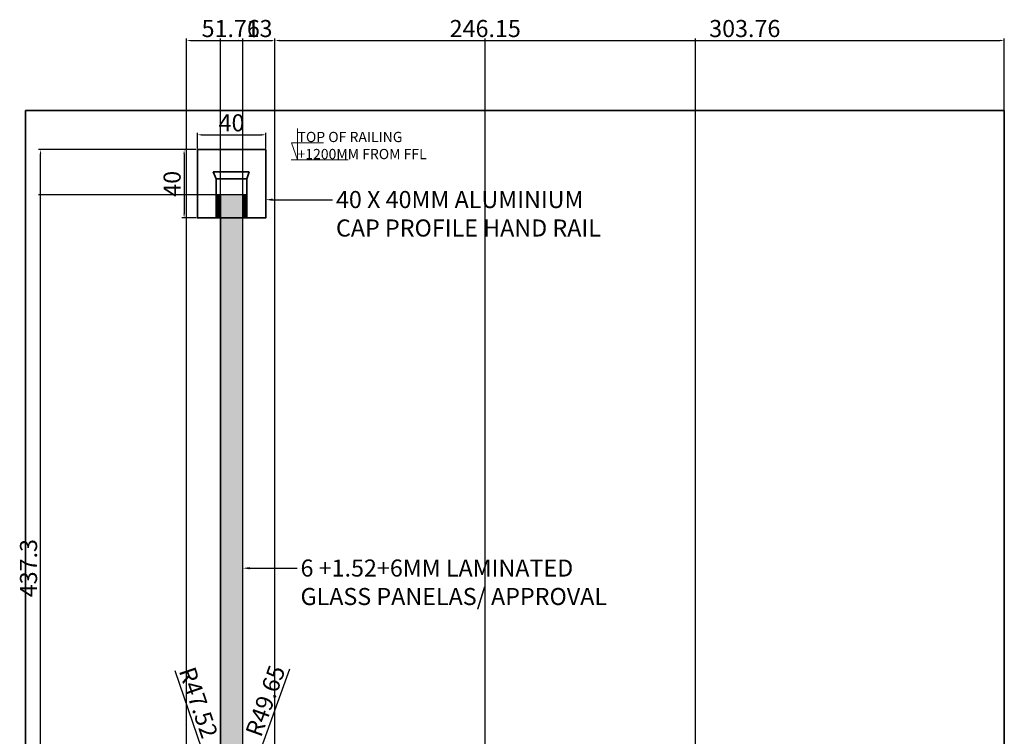
# Model space of a CAD drawing. Units: millimetres. Extents: x 1791 to 2420, y 1225 to 2361.
# Tile 4 of 4: x 1791 to 2367, y 1941 to 2361. Entities that reach past the tile are written whole.
import ezdxf
from ezdxf import colors
from ezdxf.entities.mleader import LeaderData, LeaderLine
from ezdxf.math import Vec2, Vec3

# ---------------------------------------------------------------- set-up
doc = ezdxf.new("R2010")
doc.units = ezdxf.units.MM
for name, color, linetype, lineweight in [('A-ANNO-DIMS', 2, 'Continuous', 18), ('A-ANNO-SYMB', 7, 'Continuous', 18), ('A-ANNO-TEXT', 7, 'Continuous', 18), ('A-ANNO-TTLB', 7, 'Continuous', 35), ('A-DETL-PATT', 8, 'Continuous', 13), ('A-GLAZ', 5, 'Continuous', 25), ('A-RAIL', 4, 'Continuous', 35)]:
    doc.layers.add(name, color=color, linetype=linetype, lineweight=lineweight)
doc.styles.get("Standard").update_dxf_attribs({"font": 'arial.ttf'})
doc.dimstyles.new('ISO-25', dxfattribs={"dimtxt": 10, "dimasz": 2.5, "dimexe": 1.25, "dimexo": 0.625, "dimtad": 1, "dimdec": 1, "dimtxsty": 'Standard', "dimcen": 2.5, "dimadec": 0, "dimazin": 0, "dimtfac": 1, "dimtdec": 1, "dimtmove": 0, "dimatfit": 3, "dimfxl": 1, "dimarcsym": 0})

# ---------------------------------------------------------------- blocks, each defined once
blk = doc.blocks.new('*D1')
at = {"layer": 'A-ANNO-DIMS', "color": 0, "lineweight": -2, "transparency": 16777216}
for p, q in [((1895, 2285.61), (1895, 2294.91)), ((1897.5, 2293.66), (1932.5, 2293.66)), ((1935, 2285.61), (1935, 2294.91))]:
    blk.add_line(p, q, dxfattribs=at)
at = {"layer": 'A-ANNO-DIMS', "color": 0, "transparency": 16777216}
for points in [[(1897.5, 2294.08), (1897.5, 2293.25), (1895, 2293.66)], [(1932.5, 2294.08), (1932.5, 2293.25), (1935, 2293.66)]]:
    blk.add_solid(points, dxfattribs=at)
at = {"layer": 'Defpoints', "color": 0, "transparency": 16777216}
for p in [(1935, 2293.66), (1895, 2284.98), (1935, 2284.98)]:
    blk.add_point(p, dxfattribs=at)
at = {"layer": 'A-ANNO-DIMS', "color": 0, "transparency": 16777216, "insert": (1915, 2299.39), "char_height": 10, "attachment_point": 5}
blk.add_mtext('40', dxfattribs=at)
blk = doc.blocks.new('*D2')
at = {"layer": 'A-ANNO-DIMS', "color": 0, "lineweight": -2, "transparency": 16777216}
for p, q in [((1894.37, 2284.98), (1885.99, 2284.98)), ((1887.24, 2282.48), (1887.24, 2247.48)), ((1894.37, 2244.98), (1885.99, 2244.98))]:
    blk.add_line(p, q, dxfattribs=at)
at = {"layer": 'A-ANNO-DIMS', "color": 0, "transparency": 16777216}
for points in [[(1886.82, 2282.48), (1887.66, 2282.48), (1887.24, 2284.98)], [(1886.82, 2247.48), (1887.66, 2247.48), (1887.24, 2244.98)]]:
    blk.add_solid(points, dxfattribs=at)
at = {"layer": 'Defpoints', "color": 0, "transparency": 16777216}
for p in [(1895, 2284.98), (1887.24, 2244.98), (1895, 2244.98)]:
    blk.add_point(p, dxfattribs=at)
at = {"layer": 'A-ANNO-DIMS', "color": 0, "transparency": 16777216, "insert": (1881.51, 2264.98), "char_height": 10, "attachment_point": 5, "rotation": 90}
blk.add_mtext('40', dxfattribs=at)
blk = doc.blocks.new('*D11')
at = {"layer": 'A-ANNO-DIMS', "color": 0, "lineweight": -2, "transparency": 16777216}
for p, q in [((1894.37, 2284.98), (1801.98, 2284.98)), ((1803.23, 1317.92), (1803.23, 2282.48)), ((1854.1, 1315.42), (1801.98, 1315.42))]:
    blk.add_line(p, q, dxfattribs=at)
at = {"layer": 'A-ANNO-DIMS', "color": 0, "transparency": 16777216}
for points in [[(1802.81, 2282.48), (1803.64, 2282.48), (1803.23, 2284.98)], [(1802.81, 1317.92), (1803.64, 1317.92), (1803.23, 1315.42)]]:
    blk.add_solid(points, dxfattribs=at)
at = {"layer": 'Defpoints', "color": 0, "transparency": 16777216}
for p in [(1803.23, 2284.98), (1895, 2284.98), (1854.73, 1315.42)]:
    blk.add_point(p, dxfattribs=at)
at = {"layer": 'A-ANNO-DIMS', "color": 0, "transparency": 16777216, "insert": (1797.5, 1800.2), "char_height": 10, "attachment_point": 5, "rotation": 90}
blk.add_mtext('969.6', dxfattribs=at)
blk = doc.blocks.new('*D12')
at = {"layer": 'A-ANNO-DIMS', "color": 0, "lineweight": -2, "transparency": 16777216}
for p, q in [((1908.56, 1821.87), (1908.56, 2350.12)), ((1911.06, 2348.87), (1919.06, 2348.87)), ((1921.56, 1821.87), (1921.56, 2350.12)), ((1921.56, 2348.87), (1938.7, 2348.87))]:
    blk.add_line(p, q, dxfattribs=at)
at = {"layer": 'A-ANNO-DIMS', "color": 0, "transparency": 16777216}
for points in [[(1911.06, 2349.29), (1911.06, 2348.45), (1908.56, 2348.87)], [(1919.06, 2349.29), (1919.06, 2348.45), (1921.56, 2348.87)]]:
    blk.add_solid(points, dxfattribs=at)
at = {"layer": 'Defpoints', "color": 0, "transparency": 16777216}
for p in [(1921.56, 2348.87), (1908.56, 1821.24), (1921.56, 1821.24)]:
    blk.add_point(p, dxfattribs=at)
at = {"layer": 'A-ANNO-DIMS', "color": 0, "transparency": 16777216, "insert": (1931.38, 2354.6), "char_height": 10, "attachment_point": 5}
blk.add_mtext('13', dxfattribs=at)
blk = doc.blocks.new('*D13')
at = {"layer": 'A-ANNO-DIMS', "color": 0, "lineweight": -2, "transparency": 16777216}
for p, q in [((1907.94, 2258.52), (1801.98, 2258.52)), ((1803.23, 1823.74), (1803.23, 2256.02)), ((1907.94, 1821.24), (1801.98, 1821.24))]:
    blk.add_line(p, q, dxfattribs=at)
at = {"layer": 'A-ANNO-DIMS', "color": 0, "transparency": 16777216}
for points in [[(1802.81, 2256.02), (1803.64, 2256.02), (1803.23, 2258.52)], [(1802.81, 1823.74), (1803.64, 1823.74), (1803.23, 1821.24)]]:
    blk.add_solid(points, dxfattribs=at)
at = {"layer": 'Defpoints', "color": 0, "transparency": 16777216}
for p in [(1803.23, 2258.52), (1908.56, 2258.52), (1908.56, 1821.24)]:
    blk.add_point(p, dxfattribs=at)
at = {"layer": 'A-ANNO-DIMS', "color": 0, "transparency": 16777216, "insert": (1797.49, 2039.88), "char_height": 10, "attachment_point": 5, "rotation": 90}
blk.add_mtext('437.3', dxfattribs=at)
blk = doc.blocks.new('*D15')
at = {"layer": 'A-ANNO-DIMS', "color": 0, "lineweight": -2, "transparency": 16777216}
for p, q in [((1888.61, 1928.05), (1888.61, 2350.12)), ((1891.11, 2348.87), (1937.88, 2348.87)), ((1940.38, 1928.05), (1940.38, 2350.12))]:
    blk.add_line(p, q, dxfattribs=at)
at = {"layer": 'A-ANNO-DIMS', "color": 0, "transparency": 16777216}
for points in [[(1891.11, 2349.29), (1891.11, 2348.45), (1888.61, 2348.87)], [(1937.88, 2349.29), (1937.88, 2348.45), (1940.38, 2348.87)]]:
    blk.add_solid(points, dxfattribs=at)
at = {"layer": 'Defpoints', "color": 0, "transparency": 16777216}
for p in [(1940.38, 2348.87), (1888.61, 1927.42), (1940.38, 1927.42)]:
    blk.add_point(p, dxfattribs=at)
at = {"layer": 'A-ANNO-DIMS', "color": 0, "transparency": 16777216, "insert": (1914.5, 2354.6), "char_height": 10, "attachment_point": 5}
blk.add_mtext('51.76', dxfattribs=at)
blk = doc.blocks.new('*D27')
at = {"layer": 'A-ANNO-DIMS', "color": 0, "lineweight": -2, "transparency": 16777216}
for p, q in [((1940.38, 1808.78), (1940.38, 2350.12)), ((1942.88, 2348.87), (2184.03, 2348.87)), ((2186.53, 1808.78), (2186.53, 2350.12))]:
    blk.add_line(p, q, dxfattribs=at)
at = {"layer": 'A-ANNO-DIMS', "color": 0, "transparency": 16777216}
for points in [[(1942.88, 2349.29), (1942.88, 2348.45), (1940.38, 2348.87)], [(2184.03, 2349.29), (2184.03, 2348.45), (2186.53, 2348.87)]]:
    blk.add_solid(points, dxfattribs=at)
at = {"layer": 'Defpoints', "color": 0, "transparency": 16777216}
for p in [(2186.53, 2348.87), (1940.38, 1808.15), (2186.53, 1808.15)]:
    blk.add_point(p, dxfattribs=at)
at = {"layer": 'A-ANNO-DIMS', "color": 0, "transparency": 16777216, "insert": (2063.45, 2354.6), "char_height": 10, "attachment_point": 5}
blk.add_mtext('246.15', dxfattribs=at)
blk = doc.blocks.new('*D28')
at = {"layer": 'A-ANNO-DIMS', "color": 0, "lineweight": -2, "transparency": 16777216}
for p, q in [((2063.45, 1837.62), (2063.45, 2350.12)), ((2065.95, 2348.87), (2364.72, 2348.87)), ((2367.22, 1837.62), (2367.22, 2350.12))]:
    blk.add_line(p, q, dxfattribs=at)
at = {"layer": 'A-ANNO-DIMS', "color": 0, "transparency": 16777216}
for points in [[(2065.95, 2349.29), (2065.95, 2348.45), (2063.45, 2348.87)], [(2364.72, 2349.29), (2364.72, 2348.45), (2367.22, 2348.87)]]:
    blk.add_solid(points, dxfattribs=at)
at = {"layer": 'Defpoints', "color": 0, "transparency": 16777216}
for p in [(2367.22, 2348.87), (2063.45, 1837), (2367.22, 1837)]:
    blk.add_point(p, dxfattribs=at)
at = {"layer": 'A-ANNO-DIMS', "color": 0, "transparency": 16777216, "insert": (2215.34, 2354.6), "char_height": 10, "attachment_point": 5}
blk.add_mtext('303.76', dxfattribs=at)
blk = doc.blocks.new('*D40')
at = {"layer": 'A-ANNO-DIMS', "color": 0, "lineweight": -2, "transparency": 16777216}
for p, q in [((1948.97, 1980.8), (1932.16, 1934.12)), ((1914.5, 1885.05), (1931.31, 1931.76))]:
    blk.add_line(p, q, dxfattribs=at)
at = {"layer": 'A-ANNO-DIMS', "color": 0, "transparency": 16777216}
blk.add_solid([(1931.77, 1934.26), (1932.55, 1933.98), (1931.31, 1931.76)], dxfattribs=at)
at = {"layer": 'Defpoints', "color": 0, "transparency": 16777216}
for p in [(1931.31, 1931.76), (1914.5, 1885.05)]:
    blk.add_point(p, dxfattribs=at)
at = {"layer": 'A-ANNO-DIMS', "color": 0, "transparency": 16777216, "insert": (1936.01, 1961.74), "char_height": 10, "attachment_point": 5, "rotation": 70.20087}
blk.add_mtext('R49.65', dxfattribs=at)
blk = doc.blocks.new('*D41')
at = {"layer": 'A-ANNO-DIMS', "color": 0, "lineweight": -2, "transparency": 16777216}
for p, q in [((1881.8, 1979.97), (1897.4, 1934.31)), ((1913.57, 1886.98), (1898.2, 1931.95))]:
    blk.add_line(p, q, dxfattribs=at)
at = {"layer": 'A-ANNO-DIMS', "color": 0, "transparency": 16777216}
blk.add_solid([(1897.79, 1934.45), (1897, 1934.18), (1898.2, 1931.95)], dxfattribs=at)
at = {"layer": 'Defpoints', "color": 0, "transparency": 16777216}
for p in [(1898.2, 1931.95), (1913.57, 1886.98)]:
    blk.add_point(p, dxfattribs=at)
at = {"layer": 'A-ANNO-DIMS', "color": 0, "transparency": 16777216, "insert": (1894.41, 1960.78), "char_height": 10, "attachment_point": 5, "rotation": 288.8663}
blk.add_mtext('R47.52', dxfattribs=at)

msp = doc.modelspace()

# ---------------------------------------------------------------- hatches: boundary and pattern name
at = {"layer": 'A-DETL-PATT'}
h = msp.add_hatch(dxfattribs=at)
h.set_pattern_fill('ANSI31', color=256, scale=0.2)
h.paths.add_polyline_path([(1924.019, 2258.5157), (1921.5621, 2258.5157), (1921.5621, 2244.9823), (1924.019, 2244.9823)])
h.paths.add_polyline_path([(1908.5621, 2258.5157), (1906.091, 2258.5157), (1906.091, 2244.9823), (1908.5621, 2244.9823)])
h = msp.add_hatch(color=256, dxfattribs=at)
h.dxf.hatch_style = 1
h.paths.add_polyline_path([(1921.5621, 2258.5157), (1908.5621, 2258.5157), (1908.5621, 1821.2446), (1921.5621, 1821.2446)])

# ---------------------------------------------------------------- linework, layer by layer
at = {"layer": 'A-ANNO-SYMB'}
for p, q in [((1953.6131, 2297.3684), (1953.6131, 2279.0845)), ((1950.0667, 2289.0383), (1968.711, 2289.0383)), ((1953.6131, 2279.0791), (1950.0667, 2289.0383)), ((1949.9706, 2279.0845), (1983.1824, 2279.0845))]:
    msp.add_line(p, q, dxfattribs=at)
at = {"layer": 'A-ANNO-TTLB'}
for p, q in [((1794.3467, 1287.0028), (1794.3467, 2307.8191)), ((1794.3467, 2307.8191), (2367.2176, 2307.8191)), ((2367.2176, 2307.8191), (2367.2176, 1287.0028))]:
    msp.add_line(p, q, dxfattribs=at)
at = {"layer": 'A-GLAZ'}
msp.add_lwpolyline([(1908.5621, 1821.2446), (1921.5621, 1821.2446), (1921.5621, 2258.5157), (1908.5621, 2258.5157)], close=True, dxfattribs=at)
at = {"layer": 'A-RAIL'}
for p, q in [((1904.2456, 2272.0222), (1925.3645, 2272.0222)), ((1906.091, 2267.8964), (1904.2456, 2272.0222)), ((1924.019, 2267.8964), (1925.3645, 2272.0222)), ((1908.5621, 2258.5157), (1906.091, 2258.5157)), ((1921.5621, 2258.5157), (1924.019, 2258.5157))]:
    msp.add_line(p, q, dxfattribs=at)
for points in [[(1894.9953, 2284.9823), (1934.9953, 2284.9823), (1934.9953, 2244.9823), (1894.9953, 2244.9823)], [(1906.091, 2244.9823), (1924.019, 2244.9823), (1924.019, 2267.8964), (1906.091, 2267.8964)]]:
    msp.add_lwpolyline(points, close=True, dxfattribs=at)

# ---------------------------------------------------------------- texts
at = {"layer": 'A-ANNO-TEXT', "insert": (1953.6131, 2295.3943), "char_height": 6, "attachment_point": 1}
msp.add_mtext_dynamic_manual_height_columns('TOP OF RAILING \\P+1200MM FROM FFL', width=145.2922, gutter_width=12.5, heights=[0], dxfattribs=at)

# ---------------------------------------------------------------- dimensions: what is measured, and where the dimension line sits
at = {"layer": 'A-ANNO-DIMS'}
for base, p1, p2, override, picture, middle in [((1940.378, 2348.8684), (1888.6133, 1927.4206), (1940.378, 1927.4206), {"dimdec": 2, "dimlfac": 1, "dimrnd": 0, "dimzin": 0, "dimdsep": 46, "dimlunit": 2}, '*D15', (1914.4957, 2354.5991)), ((1921.5621, 2348.8684), (1908.5621, 1821.2446), (1921.5621, 1821.2446), {"dimdec": 0, "dimlfac": 1, "dimrnd": 0, "dimzin": 0, "dimdsep": 46, "dimlunit": 2}, '*D12', (1931.3788, 2354.6025)), ((2186.5283, 2348.8684), (1940.378, 1808.1531), (2186.5283, 1808.1531), {"dimdec": 2, "dimlfac": 1, "dimrnd": 0, "dimzin": 0, "dimdsep": 46, "dimlunit": 2}, '*D27', (2063.4532, 2354.5991)), ((2367.2176, 2348.8684), (2063.4532, 1836.999), (2367.2176, 1836.999), {"dimdec": 2, "dimlfac": 1, "dimrnd": 0, "dimzin": 0, "dimdsep": 46, "dimlunit": 2}, '*D28', (2215.3354, 2354.6025)), ((1934.9953, 2293.663), (1894.9953, 2284.9823), (1934.9953, 2284.9823), {"dimclrd": 0, "dimclre": 0, "dimclrt": 0}, '*D1', (1914.9953, 2299.3937))]:
    dim = msp.add_linear_dim(base=base, p1=p1, p2=p2, dimstyle='ISO-25', override=override, dxfattribs=at)
    dim.commit()
    dim.dimension.update_dxf_attribs({"geometry": picture, "text_midpoint": middle})
for base, p1, p2, override, picture, middle in [((1803.227, 2284.9823), (1854.727, 1315.4206), (1894.9953, 2284.9823), {"dimdec": 1, "dimlfac": 1, "dimrnd": 0, "dimzin": 0, "dimdsep": 46, "dimlunit": 2}, '*D11', (1797.4963, 1800.2015)), ((1887.2408, 2244.9823), (1894.9953, 2284.9823), (1894.9953, 2244.9823), {"dimclrd": 0, "dimclre": 0, "dimclrt": 0}, '*D2', (1881.5101, 2264.9823)), ((1803.227, 2258.5157), (1908.5621, 1821.2446), (1908.5621, 2258.5157), {"dimdec": 1, "dimlfac": 1, "dimrnd": 0, "dimzin": 0, "dimdsep": 46, "dimlunit": 2}, '*D13', (1797.4929, 2039.8801))]:
    dim = msp.add_linear_dim(base=base, p1=p1, p2=p2, angle=90, dimstyle='ISO-25', override=override, dxfattribs=at)
    dim.commit()
    dim.dimension.update_dxf_attribs({"geometry": picture, "text_midpoint": middle})
for center, mpoint, picture, middle in [((1913.5708, 1886.9827), (1898.2049, 1931.9492), '*D41', (1888.9854, 1958.9291)), ((1914.4957, 1885.0453), (1931.3148, 1931.7644), '*D40', (1941.4063, 1959.7959))]:
    dim = msp.add_radius_dim(center=center, mpoint=mpoint, dimstyle='ISO-25', override={"dimdec": 2, "dimlfac": 1, "dimrnd": 0, "dimzin": 0, "dimdsep": 46, "dimlunit": 2}, dxfattribs=at)
    dim.commit()
    dim.dimension.update_dxf_attribs({"geometry": picture, "text_midpoint": middle, "dimtype": 164})

# ---------------------------------------------------------------- leaders
at = {"layer": 'A-ANNO-TEXT'}
ml = msp.add_multileader_mtext('Standard', dxfattribs=at)
ml.set_content('40 X 40MM ALUMINIUM \\PCAP PROFILE HAND RAIL', color=256)
ml.set_leader_properties()
ml.build(insert=Vec2(0, 0))
ctx = ml.context
ctx.base_point, ctx.char_height, ctx.plane_origin = Vec3(1974.1045, 2255.668), 10, Vec3(1934.9953, 2255.668)
notes = []
notes.append((ctx, [(0, (1, 1, 0), (1966.1045, 2255.668), (1, 0), 8, [(0, [(1934.9953, 2255.668)], 0, [])])]))
ctx.mtext.insert, ctx.mtext.flow_direction = Vec3(1976.1045, 2260.7533), 5
ml = msp.add_multileader_mtext('Standard', dxfattribs=at)
ml.set_content('6 +1.52+6MM LAMINATED\\PGLASS PANELAS/ APPROVAL', color=256)
ml.set_leader_properties()
ml.build(insert=Vec2(0, 0))
ctx = ml.context
ctx.base_point, ctx.char_height, ctx.plane_origin = Vec3(1953.3529, 2039.8801), 10, Vec3(1921.5621, 2039.8801)
notes.append((ctx, [(0, (1, 1, 0), (1945.3529, 2039.8801), (1, 0), 8, [(0, [(1921.5621, 2039.8801)], 0, [])])]))
ctx.mtext.insert, ctx.mtext.flow_direction = Vec3(1955.3529, 2044.9654), 5
for ctx, leaders in notes:
    for number, flags, end, landing, length, lines in leaders:
        leader = LeaderData()
        leader.index, (leader.has_last_leader_line, leader.has_dogleg_vector, leader.attachment_direction) = number, flags
        leader.last_leader_point, leader.dogleg_vector, leader.dogleg_length = Vec3(end), Vec3(landing), length
        for number, points, colour, breaks in lines:
            line = LeaderLine()
            line.index, line.vertices, line.color, line.breaks = number, Vec3.list(points), colors.encode_raw_color(colour), breaks
            leader.lines.append(line)
        ctx.leaders.append(leader)

doc.saveas('drawing.dxf')
